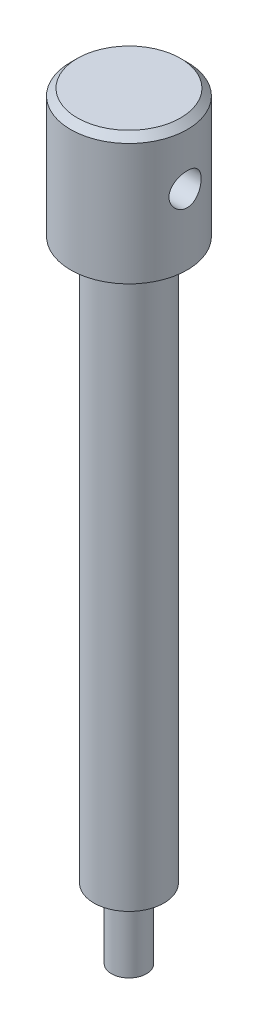
SolidWorks part; units mm, degrees
material "Plain Carbon Steel"
ref_plane "Front Plane" through (0, 0, 0) normal (0, 0, 1) x (1, 0, 0)
ref_plane "Top Plane" through (0, 0, 0) normal (0, 1, 0) x (1, 0, 0)
ref_plane "Right Plane" through (0, 0, 0) normal (1, 0, 0) x (0, 0, -1)
sketch "Tip Pin Sketch Ø6" plane through (0, 0, 0) normal (0, 1, 0) x (1, 0, 0)
  circle A0 centre (0, 0) radius 3
  dimension "D1" = 6
extrude "Tip Pin Ø6x12" add sketch "Tip Pin Sketch Ø6" along normal blind 12
sketch "Shaft Sketch Ø12" plane through (0, 12, 0) normal (0, 1, 0) x (1, 0, 0)
  circle A0 centre (0, 0) radius 6
  dimension "D1" = 12
extrude "Shaft Ø12x96" add sketch "Shaft Sketch Ø12" along normal blind 96
sketch "Head Sketch Ø20" plane through (0, 108, 0) normal (0, 1, 0) x (1, 0, 0)
  circle A0 centre (0, 0) radius 10
  dimension "D1" = 20
extrude "Head Ø20x22" add sketch "Head Sketch Ø20" along normal blind 22
sketch "Cross Hole Sketch Ø5.5" plane through (0, 0, 0) normal (1, 0, 0) x (0, 0, -1)
  line L0 (0, -1000) -> (0, 49000) construction
  circle A0 centre (0, 120) radius 2.75
  dimension "D1" = 5.5
  dimension "D2" = 12
extrude "Cross Hole Ø5.5" cut sketch "Cross Hole Sketch Ø5.5" against normal mid plane 22
chamfer "Head Chamfer 1.15x45°" distance 1.15 angle 45 1 edges at (0, 130, 10)
